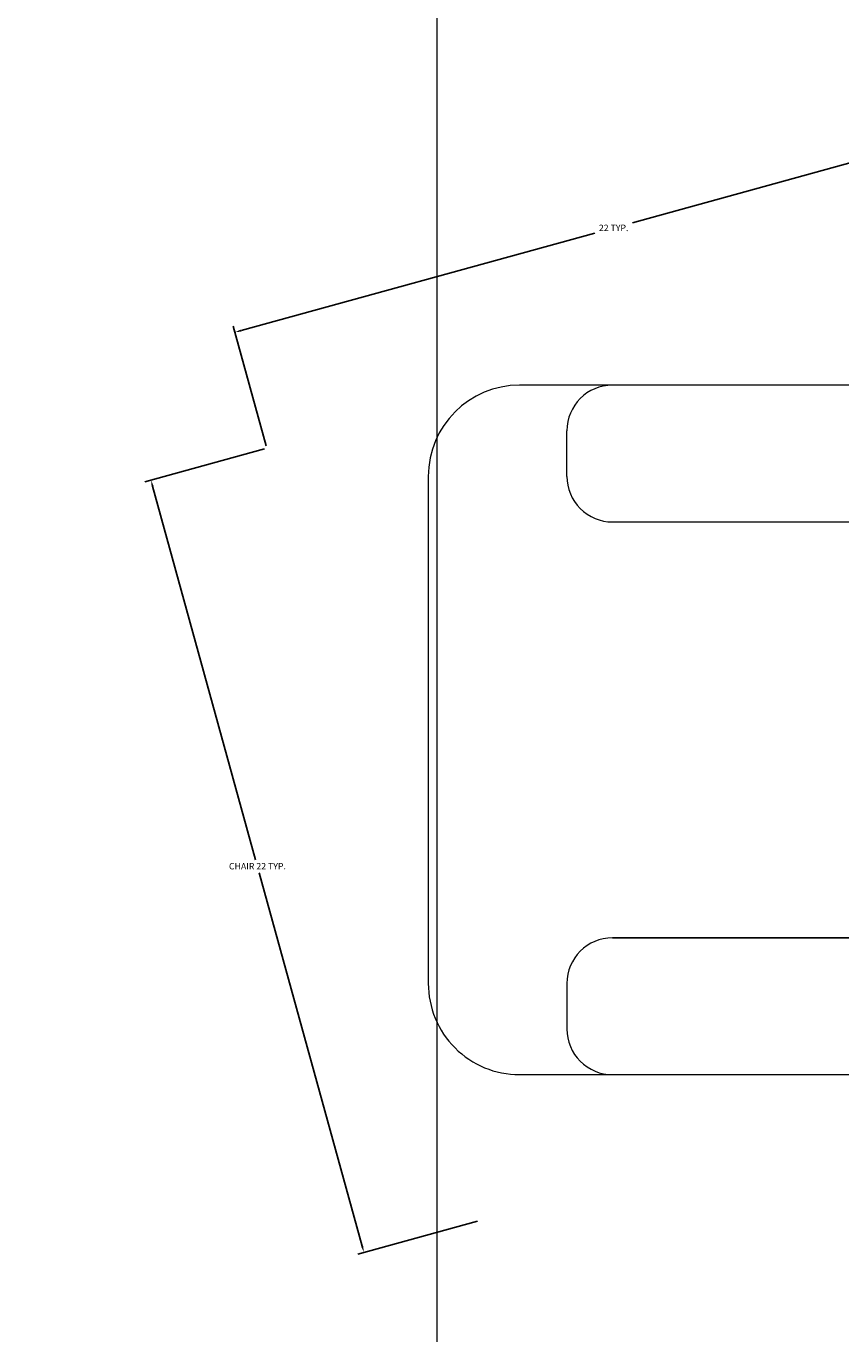
# Model space of a CAD drawing. Units: millimetres. Extents: x 27017497 to 27018854, y 7058029 to 7059154.
# Tile 16 of 91: x 27017628 to 27017651, y 7058238 to 7058275. Entities that reach past the tile are written whole.
import ezdxf

# ---------------------------------------------------------------- set-up
doc = ezdxf.new("R2010")
doc.units = ezdxf.units.MM
for name, color, linetype, lineweight in [('A-ANNO-DIMS', 2, 'Continuous', 18), ('A-FLOR-CASE', 8, 'Continuous', 20), ('A-FURN', 8, 'Continuous', 18)]:
    doc.layers.add(name, color=color, linetype=linetype, lineweight=lineweight)
doc.styles.get("Standard").update_dxf_attribs({"font": 'arial.ttf'})
doc.dimstyles.get("Standard").update_dxf_attribs({"dimtxt": 0.18, "dimasz": 0.18, "dimexe": 0.18, "dimexo": 0.0625, "dimgap": 0.09, "dimtad": 0, "dimtih": 1, "dimtoh": 1, "dimdec": 4, "dimzin": 0, "dimdsep": 46, "dimtxsty": 'Standard', "dimcen": 0.09, "dimadec": 0, "dimazin": 0, "dimtfac": 1, "dimtdec": 4, "dimtofl": 0, "dimtmove": 0, "dimatfit": 3, "dimfxl": 1, "dimtolj": 1, "dimtzin": 0, "dimarcsym": 0})

# ---------------------------------------------------------------- blocks, each defined once
blk = doc.blocks.new('CHAIR-OCCASIONAL')
for p, q in [((19.599, 18.742), (7.02, 22.21)), ((3.873, 20.423), (0.092, 6.706)), ((4.132, 6.919), (7.234, 18.169)), ((5.25, 10.974), (7.234, 18.169)), ((16.064, 15.735), (7.234, 18.169)), ((7.234, 18.169), (16.064, 15.735)), ((7.234, 18.169), (16.064, 15.735)), ((7.727, 18.033), (7.974, 17.965)), ((7.727, 18.033), (7.974, 17.965)), ((5.25, 10.974), (7.098, 17.676)), ((17.638, 16.628), (17.978, 17.862)), ((17.638, 16.628), (17.978, 17.862)), ((8.331, 17.336), (5.625, 7.52)), ((17.605, 1.878), (21.386, 15.595)), ((5.625, 7.52), (5.502, 7.072)), ((12.963, 4.485), (4.132, 6.919)), ((4.872, 6.715), (4.626, 6.783)), ((1.879, 3.558), (14.458, 0.091)), ((13.856, 2.911), (13.516, 1.678))]:
    blk.add_line(p, q)
for centre, radius, start, end in [((6.34, 19.743), 2.559, 74.5879, 164.5879), ((16.744, 18.202), 1.28, 344.5879, 74.5879), ((16.744, 18.202), 1.28, 344.5879, 74.5879), ((18.919, 16.275), 2.559, 344.5879, 74.5879), ((7.591, 17.54), 0.512, 74.5879, 164.5879), ((7.838, 17.472), 0.512, 344.5879, 74.5879), ((9.361, 16.256), 1.28, 74.5879, 164.5879), ((16.404, 16.968), 1.28, 254.5879, 344.5879), ((16.404, 16.968), 1.28, 254.5879, 344.5879), ((4.762, 7.276), 0.512, 164.5879, 254.5879), ((5.008, 7.208), 0.512, 254.5879, 344.5879), ((2.559, 6.025), 2.559, 164.5879, 254.5879), ((12.623, 3.251), 1.28, 344.5879, 74.5879), ((15.138, 2.558), 2.559, 254.5879, 344.5879), ((12.283, 2.018), 1.28, 254.5879, 344.5879)]:
    blk.add_arc(centre, radius, start, end)
blk = doc.blocks.new('*D21')
at = {"layer": 'A-ANNO-DIMS', "color": 0, "lineweight": -2, "transparency": 16777216}
for p, q in [((27017634.883, 7058262.643), (27017631.519, 7058261.716)), ((27017631.74, 7058261.59), (27017634.629, 7058251.111)), ((27017637.619, 7058240.266), (27017634.73, 7058250.745)), ((27017640.857, 7058240.972), (27017637.493, 7058240.045))]:
    blk.add_line(p, q, dxfattribs=at)
at = {"layer": 'A-ANNO-DIMS', "color": 0, "transparency": 16777216}
for points in [[(27017631.769, 7058261.598), (27017631.712, 7058261.582), (27017631.693, 7058261.764)], [(27017637.648, 7058240.274), (27017637.59, 7058240.258), (27017637.667, 7058240.092)]]:
    blk.add_solid(points, dxfattribs=at)
at = {"layer": 'Defpoints', "color": 0, "transparency": 16777216}
for p in [(27017634.943, 7058262.66), (27017640.918, 7058240.989), (27017637.667, 7058240.092)]:
    blk.add_point(p, dxfattribs=at)
at = {"layer": 'A-ANNO-DIMS', "color": 0, "transparency": 16777216, "insert": (27017634.68, 7058250.928), "char_height": 0.18, "attachment_point": 5}
blk.add_mtext('\\A1;CHAIR 22 TYP.', dxfattribs=at)
blk = doc.blocks.new('*D22')
at = {"layer": 'A-ANNO-DIMS', "color": 0, "lineweight": -2, "transparency": 16777216}
for p, q in [((27017656.18, 7058268.579), (27017655.252, 7058271.943)), ((27017655.127, 7058271.722), (27017645.203, 7058268.986)), ((27017634.221, 7058265.959), (27017644.144, 7058268.694)), ((27017634.927, 7058262.72), (27017633.999, 7058266.084))]:
    blk.add_line(p, q, dxfattribs=at)
at = {"layer": 'A-ANNO-DIMS', "color": 0, "transparency": 16777216}
for points in [[(27017655.119, 7058271.751), (27017655.135, 7058271.693), (27017655.3, 7058271.77)], [(27017634.213, 7058265.987), (27017634.229, 7058265.93), (27017634.047, 7058265.911)]]:
    blk.add_solid(points, dxfattribs=at)
at = {"layer": 'Defpoints', "color": 0, "transparency": 16777216}
for p in [(27017656.196, 7058268.519), (27017634.047, 7058265.911), (27017634.943, 7058262.66)]:
    blk.add_point(p, dxfattribs=at)
at = {"layer": 'A-ANNO-DIMS', "color": 0, "transparency": 16777216, "insert": (27017644.674, 7058268.84), "char_height": 0.18, "attachment_point": 5}
blk.add_mtext('\\A1;22 TYP.', dxfattribs=at)
blk = doc.blocks.new('*D47')
at = {"layer": 'A-ANNO-DIMS', "color": 0, "lineweight": -2, "transparency": 16777216}
for p, q in [((27017561.166, 7058294.35), (27017561.166, 7058028.6)), ((27018790.606, 7058294.35), (27018790.606, 7058028.6)), ((27017561.346, 7058028.78), (27018175.431, 7058028.78)), ((27018790.426, 7058028.78), (27018176.341, 7058028.78))]:
    blk.add_line(p, q, dxfattribs=at)
at = {"layer": 'A-ANNO-DIMS', "color": 0, "transparency": 16777216}
for points in [[(27017561.346, 7058028.81), (27017561.346, 7058028.75), (27017561.166, 7058028.78)], [(27018790.426, 7058028.81), (27018790.426, 7058028.75), (27018790.606, 7058028.78)]]:
    blk.add_solid(points, dxfattribs=at)
at = {"layer": 'Defpoints', "color": 0, "transparency": 16777216}
for p in [(27017561.166, 7058294.412), (27018790.606, 7058294.412), (27018790.606, 7058028.78)]:
    blk.add_point(p, dxfattribs=at)
at = {"layer": 'A-ANNO-DIMS', "color": 0, "transparency": 16777216, "insert": (27018175.886, 7058028.78), "char_height": 0.18, "attachment_point": 5}
blk.add_mtext('\\A1;1229.4', dxfattribs=at)
blk = doc.blocks.new('*D48')
at = {"layer": 'A-ANNO-DIMS', "color": 0, "lineweight": -2, "transparency": 16777216}
for p, q in [((27018463.498, 7058622.912), (27017497.536, 7058622.912)), ((27017497.716, 7058622.732), (27017497.716, 7058357.753)), ((27017497.716, 7058092.41), (27017497.716, 7058357.389)), ((27018555.129, 7058092.23), (27017497.536, 7058092.23))]:
    blk.add_line(p, q, dxfattribs=at)
at = {"layer": 'A-ANNO-DIMS', "color": 0, "transparency": 16777216}
for points in [[(27017497.686, 7058622.732), (27017497.746, 7058622.732), (27017497.716, 7058622.912)], [(27017497.686, 7058092.41), (27017497.746, 7058092.41), (27017497.716, 7058092.23)]]:
    blk.add_solid(points, dxfattribs=at)
at = {"layer": 'Defpoints', "color": 0, "transparency": 16777216}
for p in [(27018463.561, 7058622.912), (27017497.716, 7058092.23), (27018555.192, 7058092.23)]:
    blk.add_point(p, dxfattribs=at)
at = {"layer": 'A-ANNO-DIMS', "color": 0, "transparency": 16777216, "insert": (27017497.716, 7058357.571), "char_height": 0.18, "attachment_point": 5}
blk.add_mtext('\\A1;530.7', dxfattribs=at)

msp = doc.modelspace()

# ---------------------------------------------------------------- linework, layer by layer
at = {"layer": 'A-FLOR-CASE'}
msp.add_line((27017639.716, 7058294.412), (27017639.716, 7058207.055), dxfattribs=at)

# ---------------------------------------------------------------- block references
at = {"layer": 'A-FURN', "rotation": 195.4121391531662}
msp.add_blockref('CHAIR-OCCASIONAL', (27017655.946, 7058268.357), dxfattribs=at)

# ---------------------------------------------------------------- dimensions: what is measured, and where the dimension line sits
at = {"layer": 'A-ANNO-DIMS'}
dim = msp.add_linear_dim(base=(27017497.716, 7058092.23), p1=(27018463.561, 7058622.912), p2=(27018555.192, 7058092.23), angle=90, dimstyle='Standard', override={"dimdec": 1, "dimlfac": 1, "dimrnd": 0, "dimzin": 0, "dimdsep": 46, "dimlunit": 2}, dxfattribs=at)
dim.commit()
dim.dimension.update_dxf_attribs({"geometry": '*D48', "text_midpoint": (27017497.716, 7058357.571)})
dim = msp.add_linear_dim(base=(27018790.606, 7058028.78), p1=(27017561.166, 7058294.412), p2=(27018790.606, 7058294.412), dimstyle='Standard', override={"dimdec": 1, "dimlfac": 1, "dimrnd": 0, "dimzin": 0, "dimdsep": 46, "dimlunit": 2}, dxfattribs=at)
dim.commit()
dim.dimension.update_dxf_attribs({"geometry": '*D47', "text_midpoint": (27018175.886, 7058028.78)})
for base, p1, p2, angle, text, picture, middle in [((27017634.047, 7058265.911), (27017656.196, 7058268.519), (27017634.943, 7058262.66), 195.4121, '<> TYP.', '*D22', (27017644.674, 7058268.84)), ((27017637.667, 7058240.092), (27017634.943, 7058262.66), (27017640.918, 7058240.989), 285.4121, 'CHAIR <> TYP.', '*D21', (27017634.68, 7058250.928))]:
    dim = msp.add_linear_dim(base=base, p1=p1, p2=p2, angle=angle, text=text, dimstyle='Standard', override={"dimdec": 0, "dimlfac": 1, "dimrnd": 0, "dimzin": 0, "dimdsep": 46, "dimlunit": 2}, dxfattribs=at)
    dim.commit()
    dim.dimension.update_dxf_attribs({"geometry": picture, "text_midpoint": middle})

doc.saveas('drawing.dxf')
